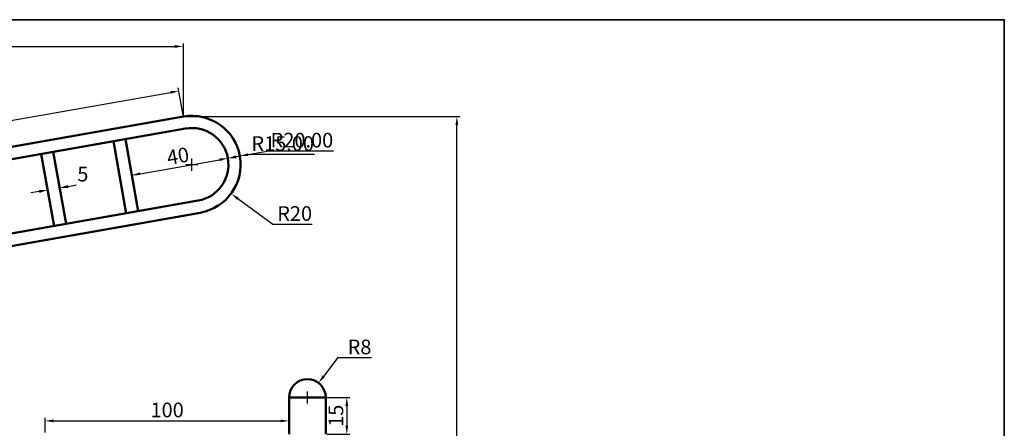
# Model space of a CAD drawing. Units: millimetres. Extents: x -71 to 780, y -41 to 454.
# Tile 4 of 4: x 376 to 780, y 287 to 454. Entities that reach past the tile are written whole.
import ezdxf

# ---------------------------------------------------------------- set-up
doc = ezdxf.new("R2010")
doc.units = ezdxf.units.MM
for name, color, linetype, lineweight in [('M-DIMS', 2, 'Continuous', 25), ('M-OUTL', 7, 'Continuous', 50), ('M-TTLB', 7, 'Continuous', 35)]:
    doc.layers.add(name, color=color, linetype=linetype, lineweight=lineweight)
doc.styles.get("Standard").update_dxf_attribs({"font": 'arial.ttf'})
doc.dimstyles.new('ISO-25', dxfattribs={"dimtxt": 6, "dimasz": 3.5, "dimexe": 1.25, "dimexo": 0.625, "dimtad": 1, "dimtoh": 1, "dimdec": 0, "dimtxsty": 'Standard', "dimcen": 2.5, "dimadec": 0, "dimazin": 0, "dimtfac": 1, "dimtdec": 0, "dimtofl": 0, "dimtmove": 0, "dimatfit": 3, "dimfxl": 1, "dimarcsym": 0})

# ---------------------------------------------------------------- blocks, each defined once
blk = doc.blocks.new('*D19')
at = {"layer": 'Defpoints', "color": 0, "transparency": 16777216}
for p in [(449.98, 375.08), (174.55, 323.28), (120.06, 316.91), (120.06, 316.91), (170.06, 316.91)]:
    blk.add_point(p, dxfattribs=at)
at = {"layer": 'M-DIMS', "color": 0, "lineweight": -2, "transparency": 16777216}
for p, q in [((170.69, 316.91), (176.17, 316.91)), ((174.81, 313.41), (190.77, 313.41))]:
    blk.add_line(p, q, dxfattribs=at)
for start, end in [(3.6562, 6.3438), (356.3438, 360)]:
    blk.add_arc((120.06, 316.91), 54.86, start, end, dxfattribs=at)
at = {"layer": 'M-DIMS', "color": 0, "transparency": 16777216}
for points in [[(174.01, 322.89), (175.16, 323.06), (174.09, 326.44)], [(175.39, 320.43), (174.23, 320.39), (174.92, 316.91)]]:
    blk.add_solid(points, dxfattribs=at)
at = {"layer": 'M-DIMS', "color": 0, "transparency": 16777216, "insert": (184.54, 317.1), "char_height": 6, "attachment_point": 5}
blk.add_mtext('10°', dxfattribs=at)
blk = doc.blocks.new('*D21')
at = {"layer": 'Defpoints', "color": 0, "transparency": 16777216}
for p in [(441.18, 424.97), (443.03, 414.48), (113.12, 356.3)]:
    blk.add_point(p, dxfattribs=at)
at = {"layer": 'M-DIMS', "color": 0, "lineweight": -2, "transparency": 16777216}
for p, q in [((114.71, 367.41), (437.73, 424.36)), ((442.92, 415.09), (440.96, 426.2)), ((113.01, 356.92), (111.05, 368.03))]:
    blk.add_line(p, q, dxfattribs=at)
at = {"layer": 'M-DIMS', "color": 0, "transparency": 16777216}
for points in [[(437.63, 424.94), (437.83, 423.79), (441.18, 424.97)], [(114.61, 367.98), (114.82, 366.83), (111.27, 366.8)]]:
    blk.add_solid(points, dxfattribs=at)
at = {"layer": 'M-DIMS', "color": 0, "transparency": 16777216, "insert": (263.76, 397.44), "char_height": 6, "attachment_point": 5, "rotation": 10}
blk.add_mtext('335', dxfattribs=at)
blk = doc.blocks.new('*D28')
at = {"layer": 'Defpoints', "color": 0, "transparency": 16777216}
for p in [(387.41, 384.36), (392.34, 385.23), (392.34, 385.23)]:
    blk.add_point(p, dxfattribs=at)
at = {"layer": 'M-DIMS', "color": 0, "lineweight": -2, "transparency": 16777216}
for p, q in [((383.97, 383.75), (380.52, 383.15)), ((387.31, 384.98), (387.2, 385.59)), ((392.23, 385.84), (392.12, 386.46)), ((395.78, 385.84), (399.23, 386.44))]:
    blk.add_line(p, q, dxfattribs=at)
at = {"layer": 'M-DIMS', "color": 0, "transparency": 16777216}
for points in [[(383.87, 384.33), (384.07, 383.18), (387.41, 384.36)], [(395.68, 386.41), (395.89, 385.26), (392.34, 385.23)]]:
    blk.add_solid(points, dxfattribs=at)
at = {"layer": 'M-DIMS', "color": 0, "transparency": 16777216, "insert": (401.85, 390.12), "char_height": 6, "attachment_point": 5}
blk.add_mtext('5', dxfattribs=at)
blk = doc.blocks.new('*D29')
at = {"layer": 'Defpoints', "color": 0, "transparency": 16777216}
for p in [(461.27, 397.38), (461.27, 397.38), (421.88, 390.44)]:
    blk.add_point(p, dxfattribs=at)
at = {"layer": 'M-DIMS', "color": 0, "lineweight": -2, "transparency": 16777216}
for p, q in [((425.33, 391.05), (457.83, 396.78)), ((461.17, 398), (461.06, 398.62)), ((421.77, 391.05), (421.67, 391.67))]:
    blk.add_line(p, q, dxfattribs=at)
at = {"layer": 'M-DIMS', "color": 0, "transparency": 16777216}
for points in [[(457.73, 397.35), (457.93, 396.2), (461.27, 397.38)], [(425.23, 391.62), (425.43, 390.47), (421.88, 390.44)]]:
    blk.add_solid(points, dxfattribs=at)
at = {"layer": 'M-DIMS', "color": 0, "transparency": 16777216, "insert": (440.94, 397.54), "char_height": 6, "attachment_point": 5, "rotation": 10}
blk.add_mtext('40', dxfattribs=at)
blk = doc.blocks.new('*D30')
at = {"layer": 'Defpoints', "color": 0, "transparency": 16777216}
for p in [(446.5, 394.78), (462.59, 382.9)]:
    blk.add_point(p, dxfattribs=at)
at = {"layer": 'M-DIMS', "color": 0, "lineweight": -2, "transparency": 16777216}
for p, q in [((446.5, 392.28), (446.5, 397.28)), ((444, 394.78), (449, 394.78)), ((479.69, 370.27), (465.41, 380.82)), ((495.82, 370.27), (479.69, 370.27))]:
    blk.add_line(p, q, dxfattribs=at)
at = {"layer": 'M-DIMS', "color": 0, "transparency": 16777216}
blk.add_solid([(465.75, 381.29), (465.06, 380.35), (462.59, 382.9)], dxfattribs=at)
at = {"layer": 'M-DIMS', "color": 0, "transparency": 16777216, "insert": (488.66, 373.96), "char_height": 6, "attachment_point": 5}
blk.add_mtext('R20', dxfattribs=at)
blk = doc.blocks.new('*D60')
at = {"layer": 'Defpoints', "color": 0, "transparency": 16777216}
for p in [(486.38, 289.73), (386.38, 284.32), (486.38, 284.32)]:
    blk.add_point(p, dxfattribs=at)
at = {"layer": 'M-DIMS', "color": 0, "lineweight": -2, "transparency": 16777216}
for p, q in [((386.38, 284.95), (386.38, 290.98)), ((486.38, 284.95), (486.38, 290.98)), ((389.88, 289.73), (482.88, 289.73))]:
    blk.add_line(p, q, dxfattribs=at)
at = {"layer": 'M-DIMS', "color": 0, "transparency": 16777216}
for points in [[(389.88, 290.31), (389.88, 289.15), (386.38, 289.73)], [(482.88, 290.31), (482.88, 289.15), (486.38, 289.73)]]:
    blk.add_solid(points, dxfattribs=at)
at = {"layer": 'M-DIMS', "color": 0, "transparency": 16777216, "insert": (436.38, 293.42), "char_height": 6, "attachment_point": 5}
blk.add_mtext('100', dxfattribs=at)
blk = doc.blocks.new('*D61')
at = {"layer": 'Defpoints', "color": 0, "transparency": 16777216}
for p in [(501.38, 299.32), (501.38, 284.32), (510.03, 284.32)]:
    blk.add_point(p, dxfattribs=at)
at = {"layer": 'M-DIMS', "color": 0, "lineweight": -2, "transparency": 16777216}
for p, q in [((502.01, 299.32), (511.28, 299.32)), ((510.03, 295.82), (510.03, 287.82)), ((502.01, 284.32), (511.28, 284.32))]:
    blk.add_line(p, q, dxfattribs=at)
at = {"layer": 'M-DIMS', "color": 0, "transparency": 16777216}
for points in [[(509.45, 295.82), (510.62, 295.82), (510.03, 299.32)], [(509.45, 287.82), (510.62, 287.82), (510.03, 284.32)]]:
    blk.add_solid(points, dxfattribs=at)
at = {"layer": 'M-DIMS', "color": 0, "transparency": 16777216, "insert": (506.34, 291.82), "char_height": 6, "attachment_point": 5, "rotation": 90}
blk.add_mtext('15', dxfattribs=at)
blk = doc.blocks.new('*D76')
at = {"layer": 'Defpoints', "color": 0, "transparency": 16777216}
for p in [(498.43, 305.29), (493.88, 299.32)]:
    blk.add_point(p, dxfattribs=at)
at = {"layer": 'M-DIMS', "color": 0, "lineweight": -2, "transparency": 16777216}
for p, q in [((506.27, 315.57), (500.55, 308.07)), ((520.1, 315.57), (506.27, 315.57)), ((491.38, 299.32), (496.38, 299.32)), ((493.88, 296.82), (493.88, 301.82))]:
    blk.add_line(p, q, dxfattribs=at)
at = {"layer": 'M-DIMS', "color": 0, "transparency": 16777216}
blk.add_solid([(500.09, 308.42), (501.02, 307.72), (498.43, 305.29)], dxfattribs=at)
at = {"layer": 'M-DIMS', "color": 0, "transparency": 16777216, "insert": (515.25, 319.26), "char_height": 6, "attachment_point": 5}
blk.add_mtext('R8', dxfattribs=at)
blk = doc.blocks.new('*D83')
at = {"layer": 'Defpoints', "color": 0, "transparency": 16777216}
for p in [(443.03, 414.48), (555.13, 414.48), (446.38, 119.32)]:
    blk.add_point(p, dxfattribs=at)
at = {"layer": 'M-DIMS', "color": 0, "lineweight": -2, "transparency": 16777216}
for p, q in [((443.65, 414.48), (556.38, 414.48)), ((555.13, 122.82), (555.13, 410.98)), ((447.01, 119.32), (556.38, 119.32))]:
    blk.add_line(p, q, dxfattribs=at)
at = {"layer": 'M-DIMS', "color": 0, "transparency": 16777216}
for points in [[(554.55, 410.98), (555.72, 410.98), (555.13, 414.48)], [(554.55, 122.82), (555.72, 122.82), (555.13, 119.32)]]:
    blk.add_solid(points, dxfattribs=at)
at = {"layer": 'M-DIMS', "color": 0, "transparency": 16777216, "insert": (551.45, 266.9), "char_height": 6, "attachment_point": 5, "rotation": 90}
blk.add_mtext('295.15', dxfattribs=at)
blk = doc.blocks.new('*D84')
at = {"layer": 'Defpoints', "color": 0, "transparency": 16777216}
for p in [(443.03, 443.23), (443.03, 414.48), (113.12, 356.3)]:
    blk.add_point(p, dxfattribs=at)
at = {"layer": 'M-DIMS', "color": 0, "lineweight": -2, "transparency": 16777216}
for p, q in [((113.12, 356.93), (113.12, 444.48)), ((443.03, 415.1), (443.03, 444.48)), ((116.62, 443.23), (439.53, 443.23))]:
    blk.add_line(p, q, dxfattribs=at)
at = {"layer": 'M-DIMS', "color": 0, "transparency": 16777216}
for points in [[(116.62, 443.81), (116.62, 442.64), (113.12, 443.23)], [(439.53, 443.81), (439.53, 442.64), (443.03, 443.23)]]:
    blk.add_solid(points, dxfattribs=at)
at = {"layer": 'M-DIMS', "color": 0, "transparency": 16777216, "insert": (278.07, 446.92), "char_height": 6, "attachment_point": 5}
blk.add_mtext('329.91', dxfattribs=at)
blk = doc.blocks.new('*D87')
at = {"layer": 'Defpoints', "color": 0, "transparency": 16777216}
for p in [(466.2, 398.25), (446.5, 394.78)]:
    blk.add_point(p, dxfattribs=at)
at = {"layer": 'M-DIMS', "color": 0, "lineweight": -2, "transparency": 16777216}
for p, q in [((478.02, 400.34), (469.65, 398.86)), ((504.61, 400.34), (478.02, 400.34)), ((446.5, 392.28), (446.5, 397.28)), ((444, 394.78), (449, 394.78))]:
    blk.add_line(p, q, dxfattribs=at)
at = {"layer": 'M-DIMS', "color": 0, "transparency": 16777216}
blk.add_solid([(469.54, 399.44), (469.75, 398.29), (466.2, 398.25)], dxfattribs=at)
at = {"layer": 'M-DIMS', "color": 0, "transparency": 16777216, "insert": (491.63, 404.03), "char_height": 6, "attachment_point": 5}
blk.add_mtext('R20.00', dxfattribs=at)
blk = doc.blocks.new('*D88')
at = {"layer": 'Defpoints', "color": 0, "transparency": 16777216}
for p in [(461.27, 397.38), (446.5, 394.78)]:
    blk.add_point(p, dxfattribs=at)
at = {"layer": 'M-DIMS', "color": 0, "lineweight": -2, "transparency": 16777216}
for p, q in [((446.5, 392.28), (446.5, 397.28)), ((470.14, 398.95), (464.72, 397.99)), ((496.73, 398.95), (470.14, 398.95)), ((444, 394.78), (449, 394.78))]:
    blk.add_line(p, q, dxfattribs=at)
at = {"layer": 'M-DIMS', "color": 0, "transparency": 16777216}
blk.add_solid([(464.62, 398.57), (464.82, 397.42), (461.27, 397.38)], dxfattribs=at)
at = {"layer": 'M-DIMS', "color": 0, "transparency": 16777216, "insert": (483.75, 402.64), "char_height": 6, "attachment_point": 5}
blk.add_mtext('R15.00', dxfattribs=at)

msp = doc.modelspace()

# ---------------------------------------------------------------- linework, layer by layer
at = {"layer": 'M-OUTL'}
for p, q in [((414.354, 404.343), (419.563, 374.798)), ((419.278, 405.211), (424.487, 375.667)), ((389.733, 400.002), (394.943, 370.457)), ((384.809, 399.133), (390.019, 369.589)), ((486.384, 284.324), (486.384, 299.324)), ((486.384, 299.324), (501.384, 299.324)), ((501.384, 299.324), (501.384, 284.324))]:
    msp.add_line(p, q, dxfattribs=at)
for points in [[(449.975, 375.084), (120.065, 316.912), (113.119, 356.304), (443.03, 414.476, -1)], [(449.107, 380.008), (124.121, 322.704), (118.911, 352.248), (443.898, 409.552, -1)]]:
    msp.add_lwpolyline(points, format="xyb", close=True, dxfattribs=at)
msp.add_arc((493.884, 299.324), 7.5, 0, 180, dxfattribs=at)
at = {"layer": 'M-TTLB'}
msp.add_lwpolyline([(779.526, -41.268), (-70.976, -41.268), (-70.976, 454.198), (779.526, 454.198)], close=True, dxfattribs=at)

# ---------------------------------------------------------------- dimensions: what is measured, and where the dimension line sits
at = {"layer": 'M-DIMS'}
for base, p1, p2, override, picture, middle in [((443.03, 443.226), (113.119, 356.304), (443.03, 414.476), {"dimdec": 2, "dimlfac": 1, "dimrnd": 0, "dimzin": 0, "dimdsep": 46, "dimlunit": 2}, '*D84', (278.074, 446.917)), ((486.384, 289.73), (386.384, 284.324), (486.384, 284.324), {"dimclrd": 0, "dimclre": 0, "dimclrt": 0}, '*D60', (436.384, 293.419))]:
    dim = msp.add_linear_dim(base=base, p1=p1, p2=p2, dimstyle='ISO-25', override=override, dxfattribs=at)
    dim.commit()
    dim.dimension.update_dxf_attribs({"geometry": picture, "text_midpoint": middle})
dim = msp.add_linear_dim(base=(441.179, 424.973), p1=(113.119, 356.304), p2=(443.03, 414.476), angle=10, dimstyle='ISO-25', override={"dimclrd": 0, "dimclre": 0, "dimclrt": 0}, dxfattribs=at)
dim.commit()
dim.dimension.update_dxf_attribs({"geometry": '*D21', "text_midpoint": (264.402, 393.802), "dimtype": 161})
for base, p1, p2, override, picture, middle in [((555.134, 414.476), (446.384, 119.324), (443.03, 414.476), {"dimdec": 2, "dimlfac": 1, "dimrnd": 0, "dimzin": 0, "dimdsep": 46, "dimlunit": 2}, '*D83', (551.446, 266.9)), ((510.033, 284.324), (501.384, 299.324), (501.384, 284.324), {"dimclrd": 0, "dimclre": 0, "dimclrt": 0}, '*D61', (506.344, 291.824))]:
    dim = msp.add_linear_dim(base=base, p1=p1, p2=p2, angle=90, dimstyle='ISO-25', override=override, dxfattribs=at)
    dim.commit()
    dim.dimension.update_dxf_attribs({"geometry": picture, "text_midpoint": middle})
for center, mpoint, override, picture, middle in [((446.503, 394.78), (466.199, 398.253), {"dimdec": 2, "dimlfac": 1, "dimrnd": 0, "dimzin": 0, "dimdsep": 46, "dimlunit": 2}, '*D87', (478.016, 400.337)), ((446.503, 394.78), (461.275, 397.385), {"dimdec": 2, "dimlfac": 1, "dimrnd": 0, "dimzin": 0, "dimdsep": 46, "dimlunit": 2}, '*D88', (470.138, 398.948)), ((446.503, 394.78), (462.591, 382.898), {"dimclrd": 0, "dimclre": 0, "dimclrt": 0}, '*D30', (488.663, 370.273)), ((493.8841, 299.324), (498.4324, 305.2875), {"dimclrd": 0, "dimclre": 0, "dimclrt": 0}, '*D76', (515.2543, 315.5686))]:
    dim = msp.add_radius_dim(center=center, mpoint=mpoint, dimstyle='ISO-25', override=override, dxfattribs=at)
    dim.commit()
    dim.dimension.update_dxf_attribs({"geometry": picture, "text_midpoint": middle, "dimtype": 164})
for p1, p2, picture, middle in [((421.882, 390.439), (461.275, 397.385), '*D29', (440.938, 397.544)), ((387.414, 384.361), (392.338, 385.229), '*D28', (401.846, 390.121))]:
    dim = msp.add_aligned_dim(p1=p1, p2=p2, distance=0, dimstyle='ISO-25', override={"dimclrd": 0, "dimclre": 0, "dimclrt": 0}, dxfattribs=at)
    dim.commit()
    dim.dimension.update_dxf_attribs({"geometry": picture, "text_midpoint": middle})
dim = msp.add_angular_dim_2l(base=(174.551, 323.28), line1=((170.063, 316.912), (120.065, 316.912)), line2=((449.975, 375.084), (120.065, 316.912)), dimstyle='ISO-25', override={"dimclrd": 0, "dimclre": 0, "dimclrt": 0}, dxfattribs=at)
dim.commit()
dim.dimension.update_dxf_attribs({"geometry": '*D19', "text_midpoint": (184.539, 317.102)})

doc.saveas('drawing.dxf')
